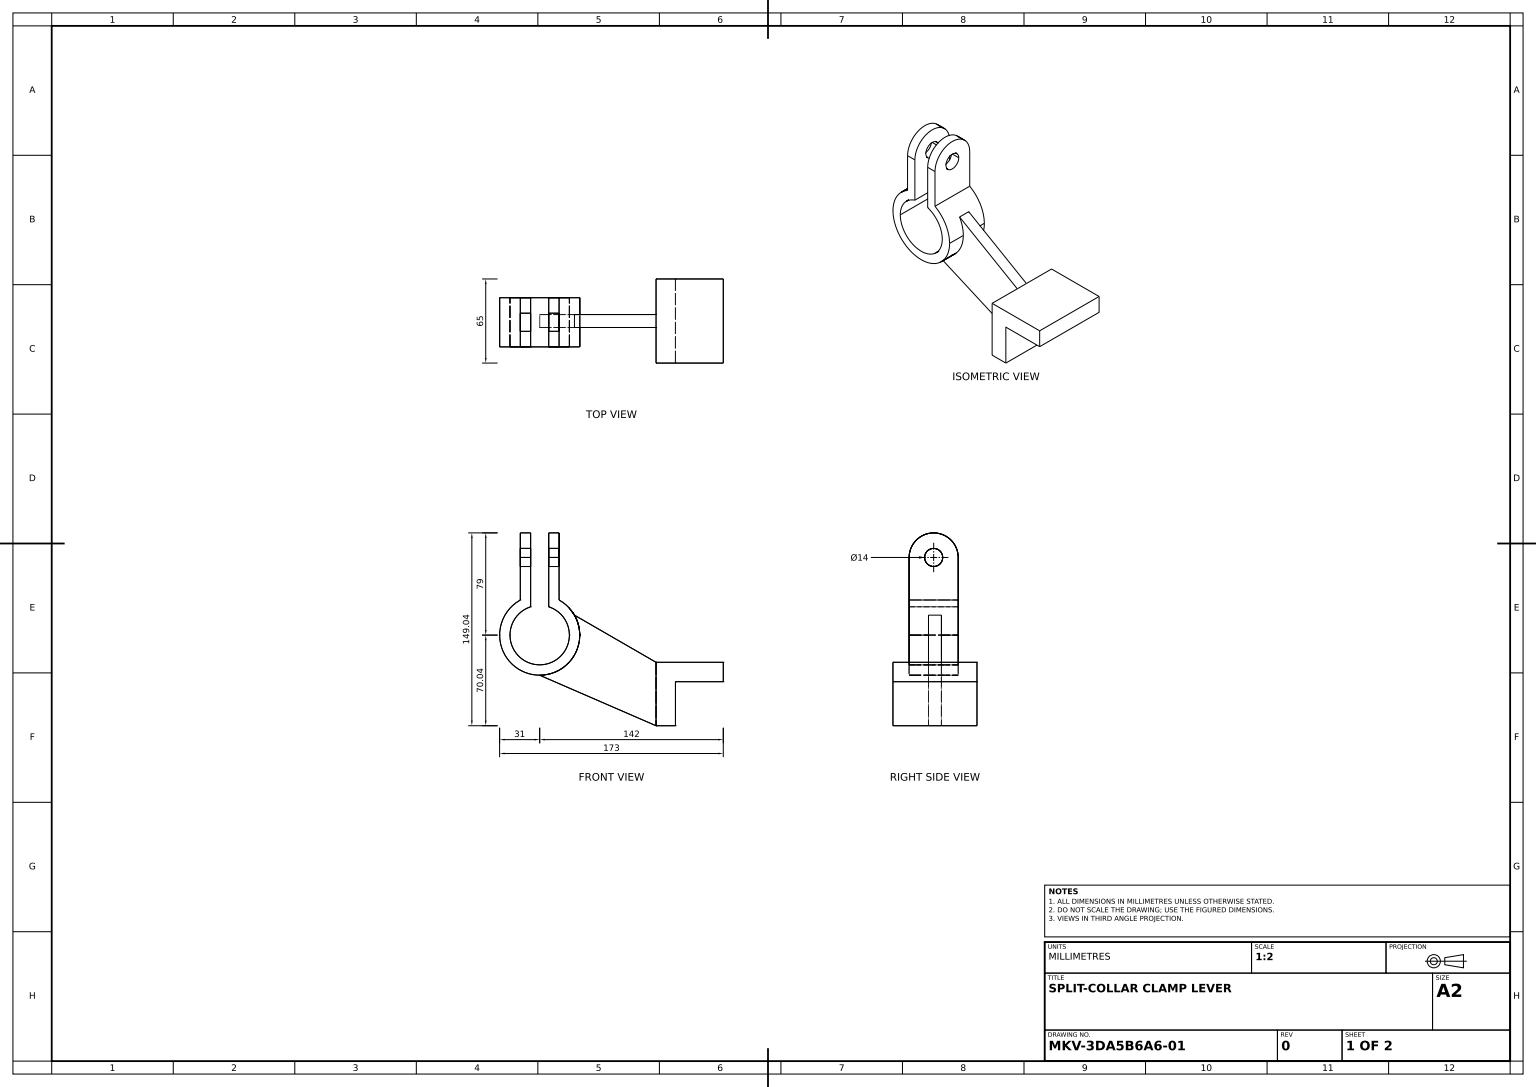
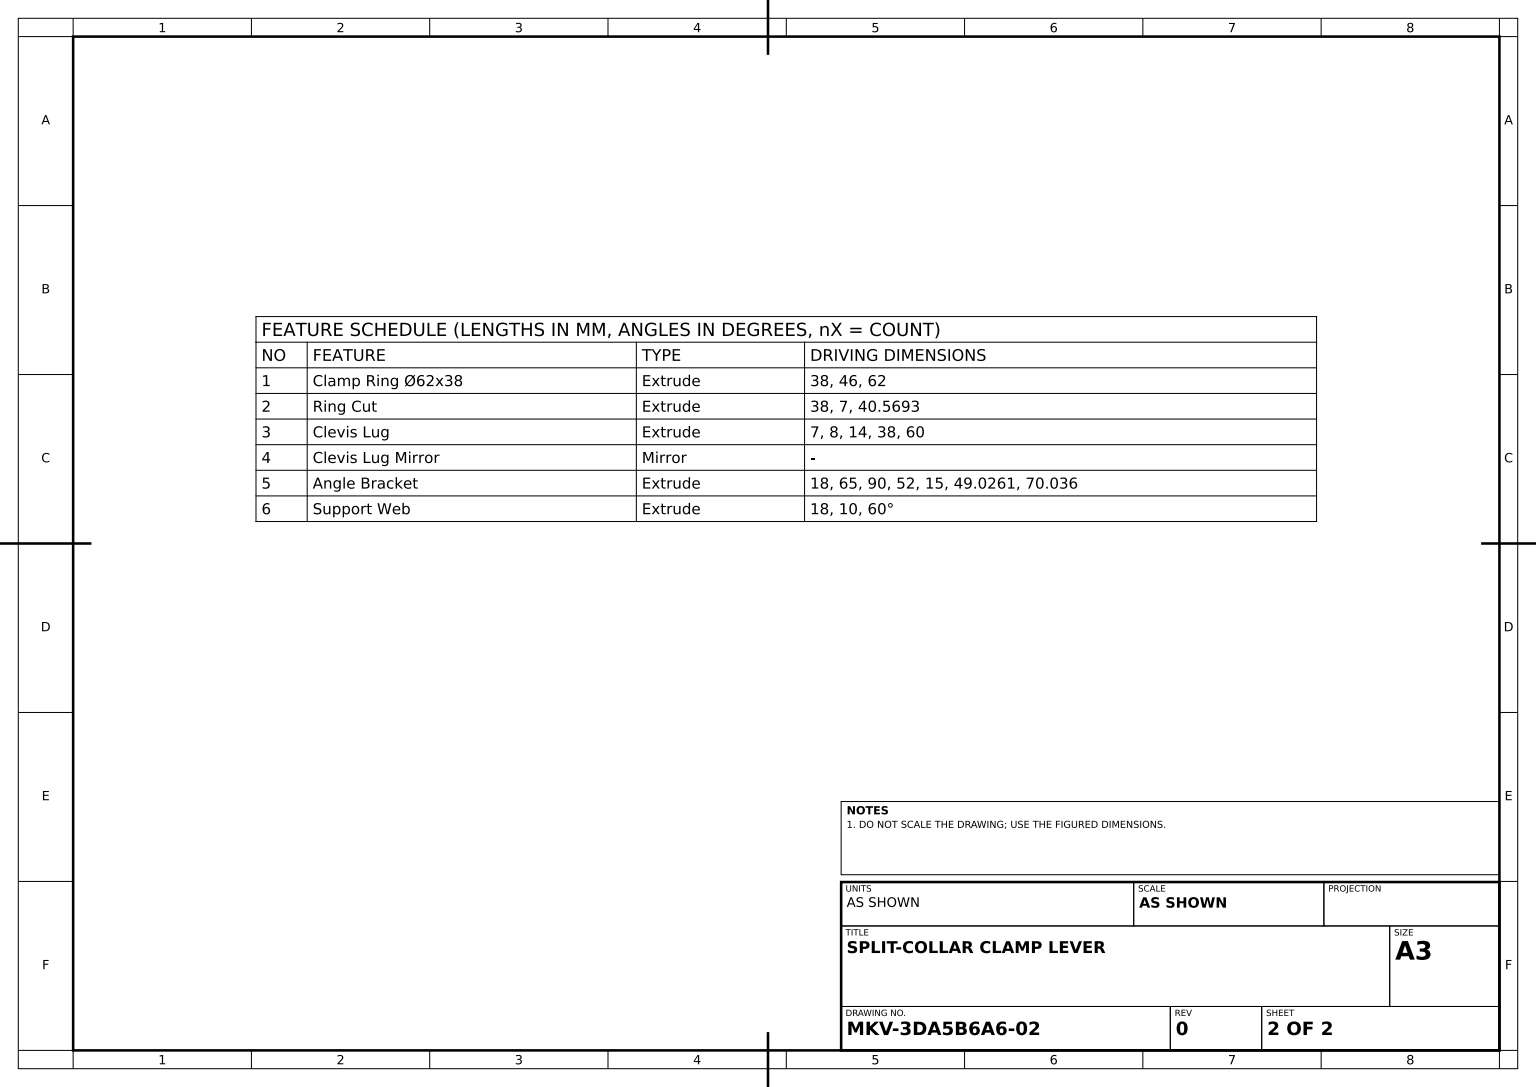
from build123d import *

# Parameters (mm, degrees)
CLAMP_RING_SKETCH_46_62_R   = 31
CLAMP_RING_SKETCH_46_62_R_2 = 23
CLAMP_RING_62X38_DEPTH      = 38
RING_CUT_DEPTH              = 38
CLEVIS_LUG_SKETCH_R         = 7
CLEVIS_LUG_DEPTH            = 8
ANGLE_BRACKET_DEPTH         = 32.5
SUPPORT_WEB_DEPTH           = 5


with BuildPart() as part:
    # Clamp Ring Sketch Ø46-Ø62 → Clamp Ring Ø62x38 (new body)
    with BuildSketch(Plane.XY):
        Circle(CLAMP_RING_SKETCH_46_62_R)
        Circle(CLAMP_RING_SKETCH_46_62_R_2, mode=Mode.SUBTRACT)
    extrude(amount=CLAMP_RING_62X38_DEPTH)

    # Ring Cut Sketch → Ring Cut (cut)
    with BuildSketch(Plane.XY.offset(38)):
        Polygon((0, 0), (-7, 0), (-7, 40.569348476), (7, 40.569348476), (7, 0), align=None)
    extrude(amount=-RING_CUT_DEPTH, mode=Mode.SUBTRACT)

    # Clevis Lug Sketch → Clevis Lug (add)
    with BuildSketch(Plane(origin=(7, 0, 0), x_dir=(0, 0, -1), z_dir=(1, 0, 0))):
        with BuildLine():
            Line((-38, 60), (-38, 21.9089023))
            Line((-38, 21.9089023), (0, 21.9089023))
            Line((0, 21.9089023), (0, 60))
            ThreePointArc((0, 60), (-19, 79), (-38, 60))
        make_face()
        with Locations((-19, 60)):
            Circle(CLEVIS_LUG_SKETCH_R, mode=Mode.SUBTRACT)
    clevis_lug = extrude(amount=CLEVIS_LUG_DEPTH)

    # Clevis Lug Mirror: Clevis Lug across plane
    add(clevis_lug.mirror(Plane(origin=(0, 0, 0), x_dir=(0, 0, 1), z_dir=(1, 0, 0))))



with BuildPart() as body_2:
    # Angle Bracket Sketch → Angle Bracket (new, symmetric)
    with BuildSketch(Plane.XY.offset(18)):
        Polygon((90, -70.036000309), (105, -70.036000309), (105, -36.009933812), (142, -36.009933812), (142, -21.009933812), (90, -21.009933812), align=None)
    extrude(amount=ANGLE_BRACKET_DEPTH, both=True)


with BuildPart() as part_1:
    add(part.part)

    add(body_2.part)  # Support Web merges body 2
    # Support Web Sketch 60deg → Support Web (add, symmetric)
    with BuildSketch(Plane.XY.offset(18)):
        with BuildLine():
            Line((90, -70.036000309), (0, -31))
            ThreePointArc((0, -31), (26.825849969, -15.536208463), (26.888515957, 15.427498489))
            Line((26.888515957, 15.427498489), (90, -21.009933812))
            Line((90, -21.009933812), (142, -21.009933812))
            Line((142, -21.009933812), (142, -36.009933812))
            Line((142, -36.009933812), (105, -36.009933812))
            Line((105, -36.009933812), (105, -70.036000309))
            Line((105, -70.036000309), (90, -70.036000309))
        make_face()
    extrude(amount=SUPPORT_WEB_DEPTH, both=True)


solid = part_1.part
